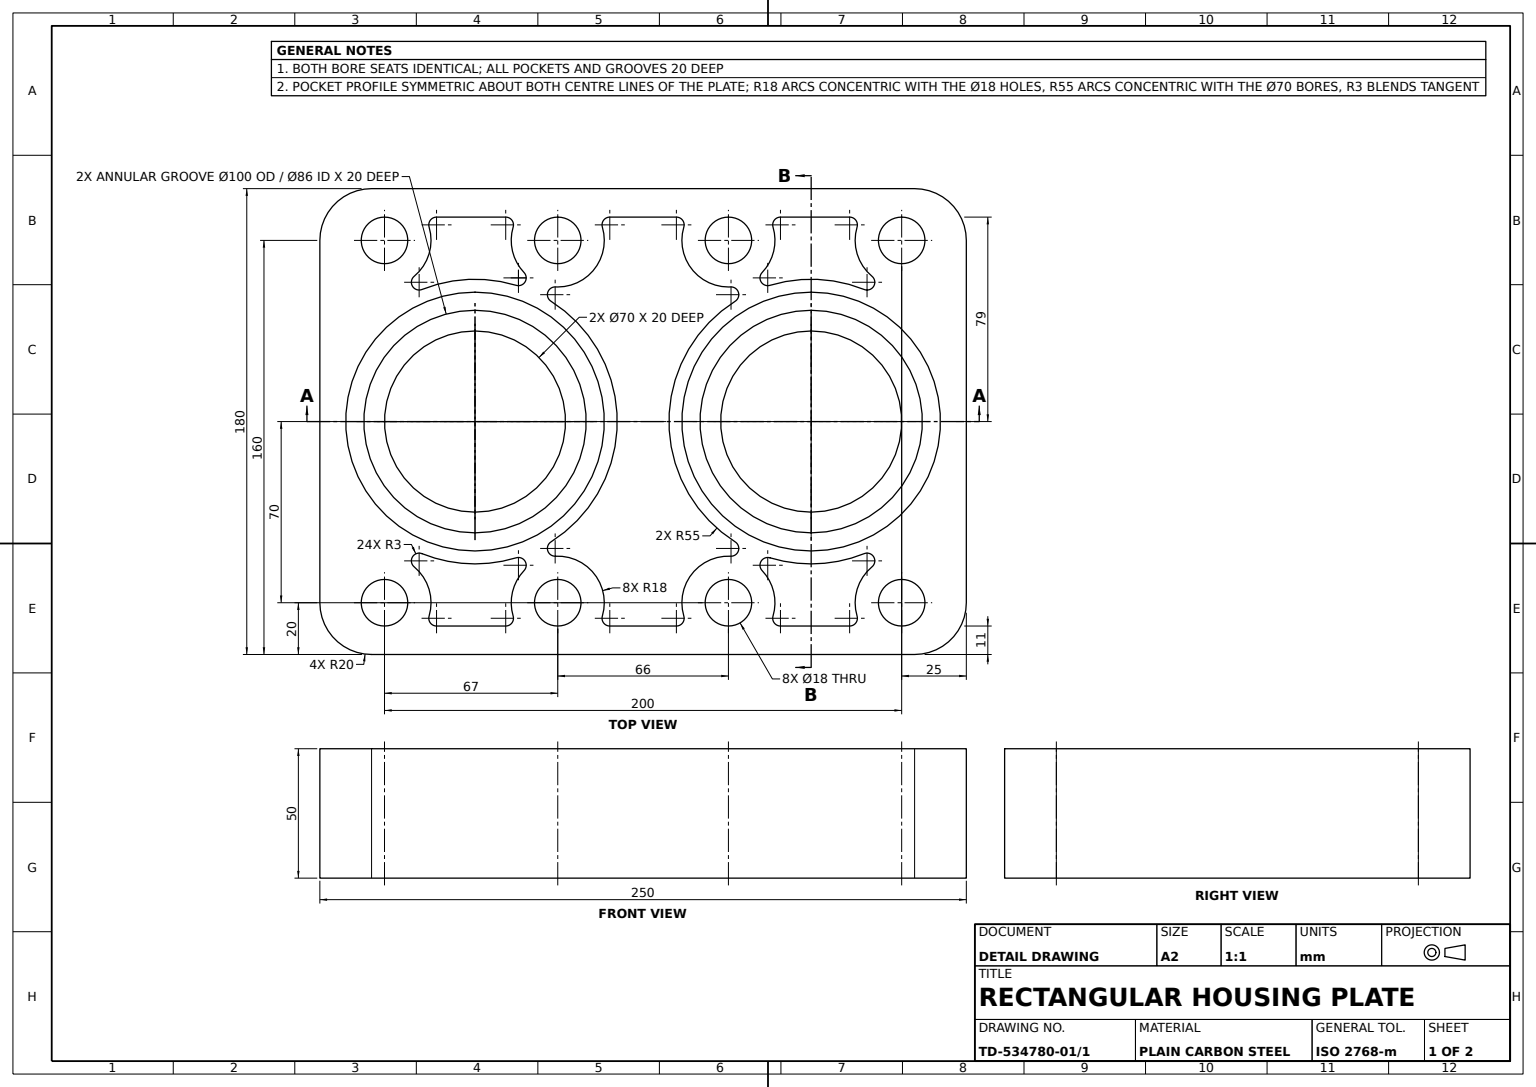
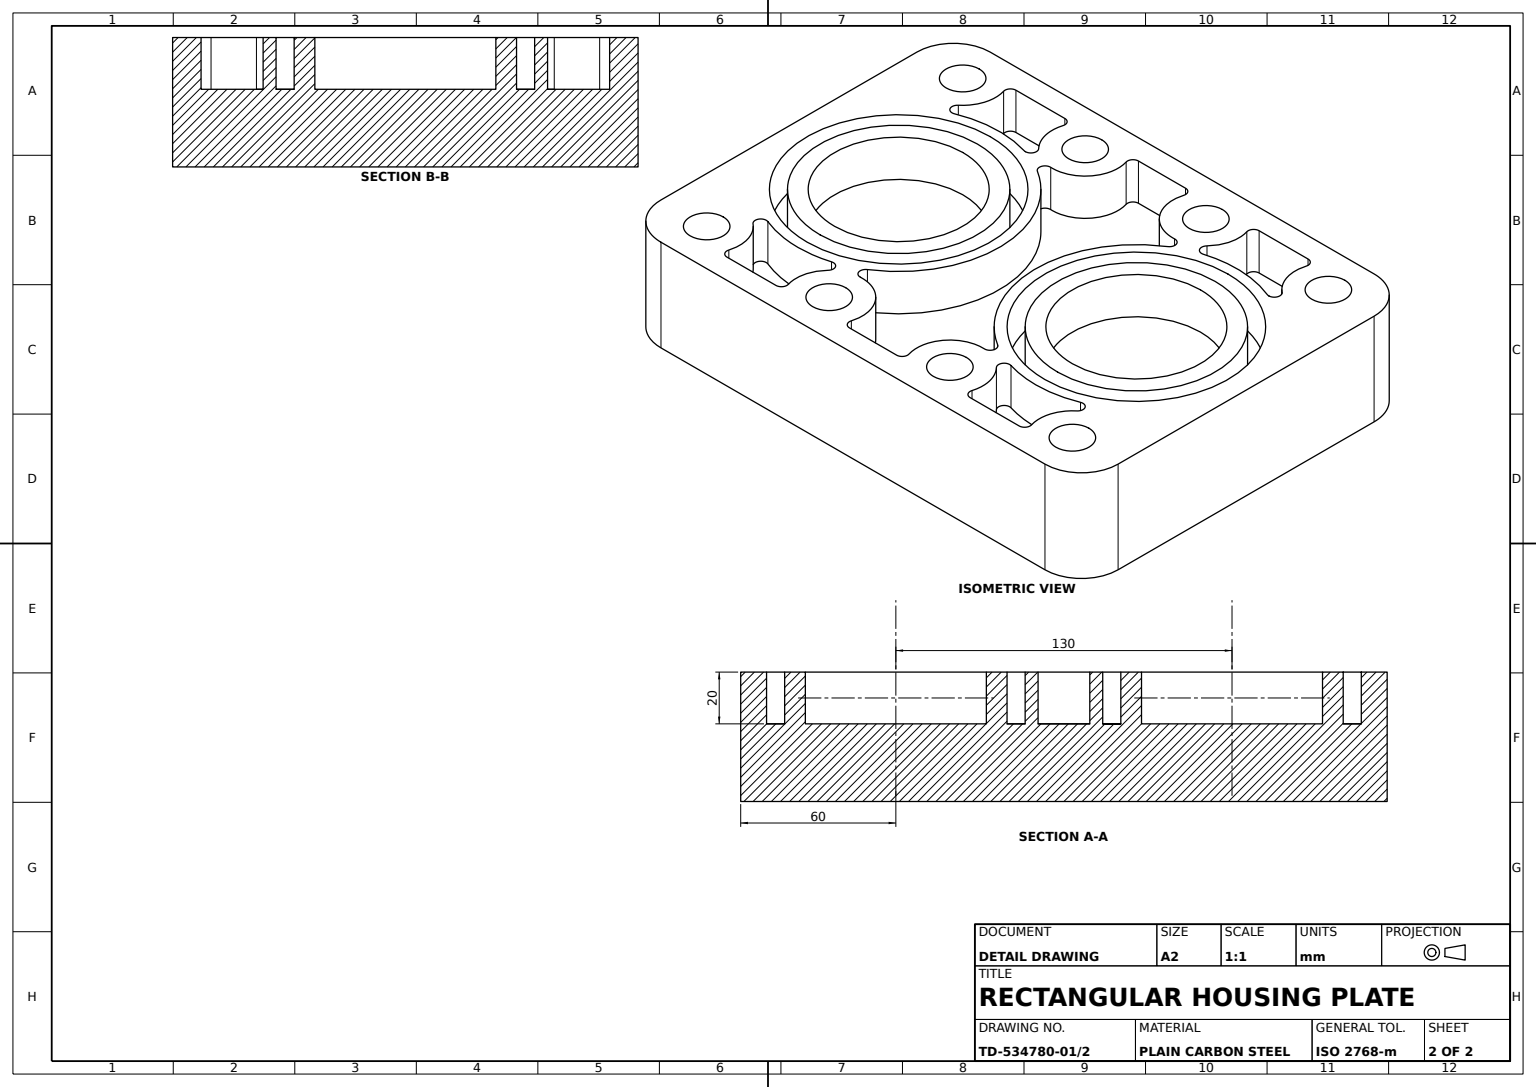
from build123d import *

# Parameters (mm, degrees)
BASE_PLATE_250X180X50_DEPTH          = 50
BORE_SEATS_AND_POCKETS_PROFILE_R     = 50
BORE_SEATS_AND_POCKETS_PROFILE_R_2   = 43
BORE_SEATS_AND_POCKETS_PROFILE_R_3   = 35
BORE_SEATS_AND_POCKETS_20_DEEP_DEPTH = 20
BOLT_HOLES_PROFILE_R                 = 9
BOLT_HOLES_8X_18_DEPTH               = 200
CORNER_ROUND_R20_A_R                 = 20
CORNER_ROUND_R20_B_R                 = 20
CORNER_ROUND_R20_C_R                 = 20
CORNER_ROUND_R20_D_R                 = 20


with BuildPart() as part:
    # Base Plate Profile → Base Plate 250x180x50 (new body)
    with BuildSketch(Plane(origin=(0, 0, 0), x_dir=(1, 0, 0), z_dir=(0, 1, 0))):
        Polygon((125, 0), (125, 90), (-125, 90), (-125, -90), (125, -90), align=None)
    extrude(amount=BASE_PLATE_250X180X50_DEPTH)

    # Bore Seats and Pockets Profile → Bore Seats and Pockets 20 Deep (cut)
    # profile 1 of 9: a face of its own
    with BuildSketch(Plane(origin=(0, 50, 0), x_dir=(1, 0, 0), z_dir=(0, 1, 0))):
        with BuildLine():
            ThreePointArc((85.489464765, 51.040981903), (67.418125523, 54.946816732), (49.07353502, 52.643591379))
            ThreePointArc((49.07353502, 52.643591379), (45.649930196, 53.942627335), (46.032701785, 57.584337142))
            ThreePointArc((46.032701785, 57.584337142), (50.502310556, 65.796534146), (50.249667255, 75.142857143))
            ThreePointArc((50.249667255, 75.142857143), (50.71926062, 77.792842914), (53.124611797, 79))
            Line((53.124611797, 79), (79.875388203, 79))
            ThreePointArc((79.875388203, 79), (82.28073938, 77.792842914), (82.750332745, 75.142857143))
            ThreePointArc((82.750332745, 75.142857143), (82.776149203, 64.771332509), (88.520347372, 56.135744681))
            ThreePointArc((88.520347372, 56.135744681), (89.185331801, 52.291224502), (85.489464765, 51.040981903))
        make_face()
    # profile 2 of 9: a face of its own
    with BuildSketch(Plane(origin=(0, 50, 0), x_dir=(1, 0, 0), z_dir=(0, 1, 0))):
        with BuildLine():
            ThreePointArc((-35.608995423, -46.488373277), (-10, 0), (-35.608995423, 46.488373277))
            ThreePointArc((-35.608995423, 46.488373277), (-36.866627296, 49.927403152), (-33.862156902, 52.020659482))
            ThreePointArc((-33.862156902, 52.020659482), (-18.829727241, 58.900298656), (-15.750332745, 75.142857143))
            ThreePointArc((-15.750332745, 75.142857143), (-15.28073938, 77.792842914), (-12.875388203, 79))
            Line((-12.875388203, 79), (0, 79))
            Line((0, 79), (12.875388203, 79))
            ThreePointArc((12.875388203, 79), (15.28073938, 77.792842914), (15.750332745, 75.142857143))
            ThreePointArc((15.750332745, 75.142857143), (18.829727241, 58.900298656), (33.862156902, 52.020659482))
            ThreePointArc((33.862156902, 52.020659482), (36.866627296, 49.927403152), (35.608995423, 46.488373277))
            ThreePointArc((35.608995423, 46.488373277), (10, 0), (35.608995423, -46.488373277))
            ThreePointArc((35.608995423, -46.488373277), (36.866627296, -49.927403152), (33.862156902, -52.020659482))
            ThreePointArc((33.862156902, -52.020659482), (18.829727241, -58.900298656), (15.750332745, -75.142857143))
            ThreePointArc((15.750332745, -75.142857143), (15.28073938, -77.792842914), (12.875388203, -79))
            Line((12.875388203, -79), (0, -79))
            Line((0, -79), (-12.875388203, -79))
            ThreePointArc((-12.875388203, -79), (-15.28073938, -77.792842914), (-15.750332745, -75.142857143))
            ThreePointArc((-15.750332745, -75.142857143), (-18.829727241, -58.900298656), (-33.862156902, -52.020659482))
            ThreePointArc((-33.862156902, -52.020659482), (-36.866627296, -49.927403152), (-35.608995423, -46.488373277))
        make_face()
    # profile 3 of 9: a face of its own
    with BuildSketch(Plane(origin=(0, 50, 0), x_dir=(1, 0, 0), z_dir=(0, 1, 0))):
        with BuildLine():
            ThreePointArc((-49.07353502, 52.643591379), (-67.418125523, 54.946816732), (-85.489464765, 51.040981903))
            ThreePointArc((-85.489464765, 51.040981903), (-89.185331801, 52.291224502), (-88.520347372, 56.135744681))
            ThreePointArc((-88.520347372, 56.135744681), (-82.776149203, 64.771332509), (-82.750332745, 75.142857143))
            ThreePointArc((-82.750332745, 75.142857143), (-82.28073938, 77.792842914), (-79.875388203, 79))
            Line((-79.875388203, 79), (-53.124611797, 79))
            ThreePointArc((-53.124611797, 79), (-50.71926062, 77.792842914), (-50.249667255, 75.142857143))
            ThreePointArc((-50.249667255, 75.142857143), (-50.502310556, 65.796534146), (-46.032701785, 57.584337142))
            ThreePointArc((-46.032701785, 57.584337142), (-45.649930196, 53.942627335), (-49.07353502, 52.643591379))
        make_face()
    # profile 4 of 9: a face of its own
    with BuildSketch(Plane(origin=(0, 50, 0), x_dir=(1, 0, 0), z_dir=(0, 1, 0))):
        with BuildLine():
            ThreePointArc((-49.07353502, -52.643591379), (-45.649930196, -53.942627335), (-46.032701785, -57.584337142))
            ThreePointArc((-46.032701785, -57.584337142), (-50.502310556, -65.796534146), (-50.249667255, -75.142857143))
            ThreePointArc((-50.249667255, -75.142857143), (-50.71926062, -77.792842914), (-53.124611797, -79))
            Line((-53.124611797, -79), (-79.875388203, -79))
            ThreePointArc((-79.875388203, -79), (-82.28073938, -77.792842914), (-82.750332745, -75.142857143))
            ThreePointArc((-82.750332745, -75.142857143), (-82.776149203, -64.771332509), (-88.520347372, -56.135744681))
            ThreePointArc((-88.520347372, -56.135744681), (-89.185331801, -52.291224502), (-85.489464765, -51.040981903))
            ThreePointArc((-85.489464765, -51.040981903), (-67.418125523, -54.946816732), (-49.07353502, -52.643591379))
        make_face()
    # profile 5 of 9: a face of its own
    with BuildSketch(Plane(origin=(0, 50, 0), x_dir=(1, 0, 0), z_dir=(0, 1, 0))):
        with BuildLine():
            ThreePointArc((49.07353502, -52.643591379), (67.418125523, -54.946816732), (85.489464765, -51.040981903))
            ThreePointArc((85.489464765, -51.040981903), (89.185331801, -52.291224502), (88.520347372, -56.135744681))
            ThreePointArc((88.520347372, -56.135744681), (82.776149203, -64.771332509), (82.750332745, -75.142857143))
            ThreePointArc((82.750332745, -75.142857143), (82.28073938, -77.792842914), (79.875388203, -79))
            Line((79.875388203, -79), (53.124611797, -79))
            ThreePointArc((53.124611797, -79), (50.71926062, -77.792842914), (50.249667255, -75.142857143))
            ThreePointArc((50.249667255, -75.142857143), (50.502310556, -65.796534146), (46.032701785, -57.584337142))
            ThreePointArc((46.032701785, -57.584337142), (45.649930196, -53.942627335), (49.07353502, -52.643591379))
        make_face()
    # profile 6 of 9: a face of its own
    with BuildSketch(Plane(origin=(0, 50, 0), x_dir=(1, 0, 0), z_dir=(0, 1, 0))):
        with Locations(Location((65, 0, 0), (0, 0, 270))):
            Circle(BORE_SEATS_AND_POCKETS_PROFILE_R)
        with Locations(Location((65, 0, 0), (0, 0, 270))):
            Circle(BORE_SEATS_AND_POCKETS_PROFILE_R_2, mode=Mode.SUBTRACT)
    # profile 7 of 9: a face of its own
    with BuildSketch(Plane(origin=(0, 50, 0), x_dir=(1, 0, 0), z_dir=(0, 1, 0))):
        with Locations(Location((65, 0, 0), (0, 0, 270))):
            Circle(BORE_SEATS_AND_POCKETS_PROFILE_R_3)
    # profile 8 of 9: a face of its own
    with BuildSketch(Plane(origin=(0, 50, 0), x_dir=(1, 0, 0), z_dir=(0, 1, 0))):
        with Locations(Location((-65, 0, 0), (0, 0, 270))):
            Circle(BORE_SEATS_AND_POCKETS_PROFILE_R)
        with Locations(Location((-65, 0, 0), (0, 0, 270))):
            Circle(BORE_SEATS_AND_POCKETS_PROFILE_R_2, mode=Mode.SUBTRACT)
    # profile 9 of 9: a face of its own
    with BuildSketch(Plane(origin=(0, 50, 0), x_dir=(1, 0, 0), z_dir=(0, 1, 0))):
        with Locations(Location((-65, 0, 0), (0, 0, 270))):
            Circle(BORE_SEATS_AND_POCKETS_PROFILE_R_3)
    extrude(amount=-BORE_SEATS_AND_POCKETS_20_DEEP_DEPTH, mode=Mode.SUBTRACT)

    # Bolt Holes Profile → Bolt Holes 8xØ18 (cut)
    with BuildSketch(Plane(origin=(0, 50, 0), x_dir=(1, 0, 0), z_dir=(0, 1, 0))):
        with Locations(Location((100, -70, 0), (0, 0, 270))):
            Circle(BOLT_HOLES_PROFILE_R)
        with Locations(Location((33, -70, 0), (0, 0, 270))):
            Circle(BOLT_HOLES_PROFILE_R)
        with Locations(Location((-33, -70, 0), (0, 0, 270))):
            Circle(BOLT_HOLES_PROFILE_R)
        with Locations(Location((-100, -70, 0), (0, 0, 270))):
            Circle(BOLT_HOLES_PROFILE_R)
        with Locations(Location((-100, 70, 0), (0, 0, 270))):
            Circle(BOLT_HOLES_PROFILE_R)
        with Locations(Location((-33, 70, 0), (0, 0, 270))):
            Circle(BOLT_HOLES_PROFILE_R)
        with Locations(Location((33, 70, 0), (0, 0, 270))):
            Circle(BOLT_HOLES_PROFILE_R)
        with Locations(Location((100, 70, 0), (0, 0, 270))):
            Circle(BOLT_HOLES_PROFILE_R)
    extrude(amount=-BOLT_HOLES_8X_18_DEPTH, mode=Mode.SUBTRACT)

    # Corner Round R20 A
    corner_round_r20_a_edges = [part.edges().sort_by_distance(p)[0] for p in [
        (-125, 25, 90),
    ]]
    fillet(corner_round_r20_a_edges, radius=CORNER_ROUND_R20_A_R)

    # Corner Round R20 B
    corner_round_r20_b_edges = [part.edges().sort_by_distance(p)[0] for p in [
        (-125, 25, -90),
    ]]
    fillet(corner_round_r20_b_edges, radius=CORNER_ROUND_R20_B_R)

    # Corner Round R20 C
    corner_round_r20_c_edges = [part.edges().sort_by_distance(p)[0] for p in [
        (125, 25, -90),
    ]]
    fillet(corner_round_r20_c_edges, radius=CORNER_ROUND_R20_C_R)

    # Corner Round R20 D
    corner_round_r20_d_edges = [part.edges().sort_by_distance(p)[0] for p in [
        (125, 25, 90),
    ]]
    fillet(corner_round_r20_d_edges, radius=CORNER_ROUND_R20_D_R)


solid = part.part
